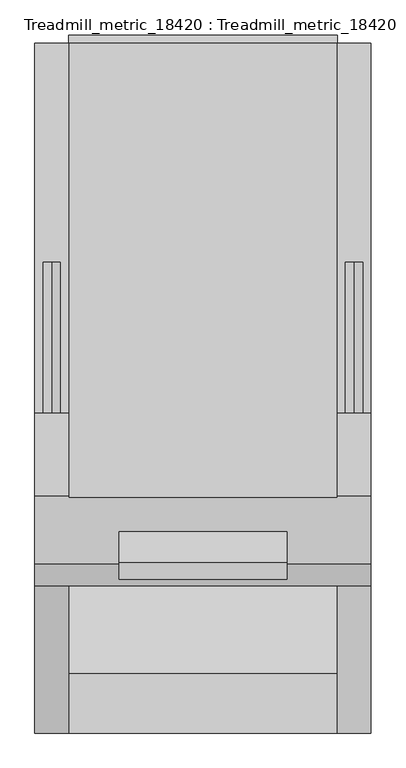
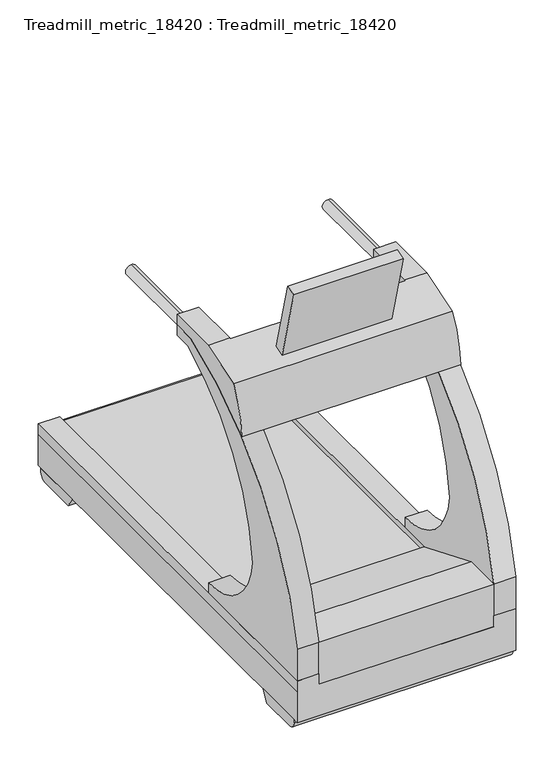
"""IFC4 building model written with IfcOpenShell, lengths in millimetres: proxy geometry, Treadmill_metric_18420 : Treadmill_metric_18420."""

from ifc_helpers import new_model, si_unit, point, frame, frame_2d, origin, place, context, project, spatial, polyline, circle_curve, trimmed, segment, composite_curve, outline, extrude, source, transform, mapped, element, save
from ifc_brep_helpers import plane_surface, cylinder_surface, revolved_surface, advanced_brep


def treadmill_metric_18420_treadmill_metric_18420_532483b1(model_context):
    return source(origin(), model_context, "Body", "SolidModel", [
        extrude(outline(composite_curve([segment(polyline([(1812.0655035, 0.0), (1781.1010673, 50.8), (2028.6449893, 50.8), (2028.6449893, 38.1)]), True, "CONTINUOUS"), segment(trimmed(circle_curve(frame_2d((1990.5449893, 38.1)), 38.1), [point((2028.6449893, 38.1))], [point((1990.5449893, 0.0))], False, "CARTESIAN"), True, "CONTINUOUS"), segment(polyline([(1990.5449893, 0.0), (1812.0655035, 0.0)]), True, "CONTINUOUS")], self_intersect=False)), frame((-136.4, 0.0, 0.0), z_axis=(1.0, 0.0, 0.0), x_axis=(0.0, 1.0, 0.0)), (0.0, 0.0, 1.0), 1000.0),
        extrude(outline(composite_curve([segment(polyline([(237.9344965, 0.0), (59.4550107, 0.0)]), True, "CONTINUOUS"), segment(trimmed(circle_curve(frame_2d((59.4550107, 38.1)), 38.1), [point((59.4550107, 0.0))], [point((21.3550107, 38.1))], False, "CARTESIAN"), True, "CONTINUOUS"), segment(polyline([(21.3550107, 38.1), (21.3550107, 50.8), (268.8989327, 50.8), (237.9344965, 0.0)]), True, "CONTINUOUS")], self_intersect=False)), frame((-136.4, 0.0, 0.0), z_axis=(1.0, 0.0, 0.0), x_axis=(0.0, 1.0, 0.0)), (0.0, 0.0, 1.0), 1000.0),
        extrude(outline(composite_curve([segment(trimmed(circle_curve(frame_2d((1371.6, -86.4)), 25.4), [point((1397.0, -86.4))], [point((1346.2, -86.4))], False, "CARTESIAN"), True, "CONTINUOUS"), segment(trimmed(circle_curve(frame_2d((1371.6, -86.4)), 25.4), [point((1346.2, -86.4))], [point((1397.0, -86.4))], False, "CARTESIAN"), True, "CONTINUOUS")], self_intersect=False)), frame((0.0, 950.0, 0.0), z_axis=(0.0, 1.0, 0.0), x_axis=(0.0, 0.0, 1.0)), (0.0, 0.0, 1.0), 450.0),
        extrude(outline(composite_curve([segment(trimmed(circle_curve(frame_2d((1371.6, 813.6)), 25.4), [point((1397.0, 813.6))], [point((1346.2, 813.6))], False, "CARTESIAN"), True, "CONTINUOUS"), segment(trimmed(circle_curve(frame_2d((1371.6, 813.6)), 25.4), [point((1346.2, 813.6))], [point((1397.0, 813.6))], False, "CARTESIAN"), True, "CONTINUOUS")], self_intersect=False)), frame((0.0, 950.0, 0.0), z_axis=(0.0, 1.0, 0.0), x_axis=(0.0, 0.0, 1.0)), (0.0, 0.0, 1.0), 450.0),
        extrude(outline(polyline([(200.0, -36.4), (250.8, -36.4), (250.8, -136.4), (200.0, -136.4), (50.8, -136.4), (50.8, 863.6), (200.0, 863.6), (250.8, 863.6), (250.8, 763.6), (200.0, 763.6), (200.0, -36.4)])), frame((0.0, 0.0, 0.0), z_axis=(0.0, 1.0, 0.0), x_axis=(0.0, 0.0, 1.0)), (0.0, 0.0, 1.0), 2050.0),
        extrude(outline(polyline([(550.0, 200.0), (0.0, 200.0), (0.0, 404.8), (177.8, 404.8), (550.0, 250.8), (550.0, 200.0)])), frame((-36.4, 0.0, 0.0), z_axis=(1.0, 0.0, 0.0), x_axis=(0.0, 1.0, 0.0)), (0.0, 0.0, 1.0), 800.0),
        extrude(outline(composite_curve([segment(polyline([(177.8, 200.0), (177.8, 225.4), (2050.0, 225.4)]), True, "CONTINUOUS"), segment(trimmed(circle_curve(frame_2d((2050.0, 200.0)), 25.4), [point((2050.0, 225.4))], [point((2050.0, 174.6))], False, "CARTESIAN"), True, "CONTINUOUS"), segment(polyline([(2050.0, 174.6), (2050.0, 200.0), (177.8, 200.0)]), True, "CONTINUOUS")], self_intersect=False)), frame((-36.4, 0.0, 0.0), z_axis=(1.0, 0.0, 0.0), x_axis=(0.0, 1.0, 0.0)), (0.0, 0.0, 1.0), 800.0),
        extrude(outline(composite_curve([segment(trimmed(circle_curve(frame_2d((1270.26111, 180.7492061)), 1289.8690034), [point((0.0, 404.8))], [point((840.7310736, 1397.0))], False, "CARTESIAN"), True, "CONTINUOUS"), segment(polyline([(840.7310736, 1397.0), (950.0, 1397.0), (950.0, 1346.2), (866.2507507, 1346.2)]), True, "CONTINUOUS"), segment(trimmed(circle_curve(frame_2d((1241.6021331, 534.0275676)), 894.7137644), [point((866.2507507, 1346.2))], [point((350.031958, 608.9631601))], True, "CARTESIAN"), True, "CONTINUOUS"), segment(trimmed(circle_curve(frame_2d((693.253891, 647.739532)), 345.4054174), [point((350.031958, 608.9631601))], [point((700.0, 302.4))], True, "CARTESIAN"), True, "CONTINUOUS"), segment(polyline([(700.0, 302.4), (700.0, 250.8), (0.0, 250.8), (0.0, 404.8)]), True, "CONTINUOUS")], self_intersect=False)), frame((-136.4, 0.0, 0.0), z_axis=(1.0, 0.0, 0.0), x_axis=(0.0, 1.0, 0.0)), (0.0, 0.0, 1.0), 100.0),
        extrude(outline(composite_curve([segment(trimmed(circle_curve(frame_2d((1270.26111, 180.7492061)), 1289.8690034), [point((0.0, 404.8))], [point((840.7310736, 1397.0))], False, "CARTESIAN"), True, "CONTINUOUS"), segment(polyline([(840.7310736, 1397.0), (950.0, 1397.0), (950.0, 1346.2), (866.2507507, 1346.2)]), True, "CONTINUOUS"), segment(trimmed(circle_curve(frame_2d((1241.6021331, 534.0275676)), 894.7137644), [point((866.2507507, 1346.2))], [point((350.031958, 608.9631601))], True, "CARTESIAN"), True, "CONTINUOUS"), segment(trimmed(circle_curve(frame_2d((693.253891, 647.739532)), 345.4054174), [point((350.031958, 608.9631601))], [point((700.0, 302.4))], True, "CARTESIAN"), True, "CONTINUOUS"), segment(polyline([(700.0, 302.4), (700.0, 250.8), (0.0, 250.8), (0.0, 404.8)]), True, "CONTINUOUS")], self_intersect=False)), frame((763.6, 0.0, 0.0), z_axis=(1.0, 0.0, 0.0), x_axis=(0.0, 1.0, 0.0)), (0.0, 0.0, 1.0), 100.0),
        advanced_brep(
        [(-136.4, 704.6599613, 1447.8), (-136.4, 950.0, 1447.8), (-136.4, 950.0, 1397.0), (-136.4, 840.7310736, 1397.0), (-136.4, 437.6082985, 1165.8640934), (-136.4, 501.9732306, 1384.2786219), (863.6, 704.6599613, 1447.8), (863.6, 501.9732306, 1384.2786219), (863.6, 437.6082985, 1165.8640934), (863.6, 840.7310736, 1397.0), (863.6, 950.0, 1397.0), (863.6, 950.0, 1447.8), (-36.4, 704.6599613, 1447.8), (-36.4, 950.0, 1447.8), (763.6, 950.0, 1447.8), (763.6, 704.6599613, 1447.8), (-36.4, 950.0, 1397.0), (763.6, 950.0, 1397.0), (-36.4, 840.7310736, 1397.0), (763.6, 840.7310736, 1397.0), (-36.4, 700.0, 1337.7126075), (763.6, 700.0, 1337.7126075), (763.6, 700.0, 1446.3395829), (-36.4, 700.0, 1446.3395829)],
        [
            (0, 1),
            (1, 2),
            (2, 3),
            (3, 4, circle_curve(frame((-136.4, 1270.26111, 180.7492061), z_axis=(1.0, 0.0, 0.0), x_axis=(0.0, 0.0, -1.0)), 1289.8690034)),
            (4, 5, circle_curve(frame((-136.4, 867.4146977, 1157.894915), z_axis=(-1.0, 0.0, 0.0), x_axis=(0.0, 0.0, -1.0)), 429.8802724)),
            (5, 0),
            (6, 7),
            (7, 8, circle_curve(frame((863.6, 867.4146977, 1157.894915), z_axis=(1.0, 0.0, 0.0), x_axis=(0.0, 0.0, -1.0)), 429.8802724)),
            (8, 9, circle_curve(frame((863.6, 1270.26111, 180.7492061), z_axis=(-1.0, 0.0, 0.0), x_axis=(0.0, 0.0, -1.0)), 1289.8690034)),
            (9, 10),
            (10, 11),
            (11, 6),
            (0, 12),
            (12, 13),
            (13, 1),
            (11, 14),
            (14, 15),
            (15, 6),
            (13, 16),
            (16, 2),
            (10, 17),
            (17, 14),
            (16, 18),
            (18, 3),
            (9, 19),
            (19, 17),
            (18, 20, circle_curve(frame((-36.4, 1270.26111, 180.7492061), z_axis=(1.0, 0.0, 0.0), x_axis=(0.0, 0.0, -1.0)), 1289.8690034)),
            (20, 21),
            (21, 19, circle_curve(frame((763.6, 1270.26111, 180.7492061), z_axis=(-1.0, 0.0, 0.0), x_axis=(0.0, 0.0, -1.0)), 1289.8690034)),
            (8, 4),
            (7, 5),
            (15, 22),
            (22, 23),
            (23, 12),
            (23, 20),
            (22, 21),
        ],
        [
            plane_surface(frame((-136.4, 1051.6662291, 1447.8), z_axis=(-1.0, 0.0, 0.0), x_axis=(0.0, 1.0, 0.0))),
            plane_surface(frame((863.6, 1051.6662291, 1447.8), z_axis=(1.0, 0.0, 0.0), x_axis=(0.0, -1.0, 0.0))),
            plane_surface(frame((-136.4, 704.6599613, 1447.8), z_axis=(0.0, 0.0, 1.0), x_axis=(1.0, 0.0, 0.0))),
            plane_surface(frame((-136.4, 950.0, 1447.8), z_axis=(0.0, 1.0, 0.0), x_axis=(1.0, 0.0, 0.0))),
            plane_surface(frame((-136.4, 950.0, 1397.0), z_axis=(0.0, 0.0, -1.0), x_axis=(1.0, 0.0, 0.0))),
            revolved_surface(polyline([(863.6, 1270.26111, -1109.1197973), (-136.39999999999998, 1270.26111, -1109.1197973)]), (863.6, 1270.26111, 180.7492061), (1.0, 0.0, 0.0)),
            cylinder_surface(frame((863.6, 867.4146977, 1157.894915), z_axis=(-1.0, 0.0, 0.0), x_axis=(0.0, 0.0, -1.0)), 429.8802724),
            plane_surface(frame((-136.4, 501.9732306, 1384.2786219), z_axis=(0.0, -0.29905454025397277, 0.9542360200461336), x_axis=(1.0, 0.0, 0.0))),
            plane_surface(frame((-36.4, 950.0, 1500.0), z_axis=(1.0, 0.0, 0.0), x_axis=(0.0, 0.0, -1.0))),
            plane_surface(frame((-36.4, 700.0, 1500.0), z_axis=(0.0, 1.0, 0.0), x_axis=(0.0, 0.0, -1.0))),
            plane_surface(frame((763.6, 700.0, 1500.0), z_axis=(-1.0, 0.0, 0.0), x_axis=(0.0, 0.0, -1.0))),
        ],
        [
            (0, [[1, 2, 3, 4, 5, 6]]),
            (1, [[7, 8, 9, 10, 11, 12]]),
            (2, [[-1, 13, 14, 15]]),
            (2, [[-12, 16, 17, 18]]),
            (3, [[-2, -15, 19, 20]]),
            (3, [[-11, 21, 22, -16]]),
            (4, [[-3, -20, 23, 24]]),
            (4, [[-10, 25, 26, -21]]),
            (5, [[-4, -24, 27, 28, 29, -25, -9, 30]]),
            (6, [[-5, -30, -8, 31]]),
            (7, [[-6, -31, -7, -18, 32, 33, 34, -13]]),
            (8, [[35, -27, -23, -19, -14, -34]]),
            (9, [[-35, -33, 36, -28]]),
            (10, [[-36, -32, -17, -22, -26, -29]]),
        ],
    ),
        extrude(outline(polyline([(0.0, -50.0), (0.0, 0.0), (500.0, 0.0), (500.0, -50.0), (0.0, -50.0)])), frame((113.6, 598.7271501, 1417.845423), z_axis=(0.0, -0.25881904510252135, 0.9659258262890681), x_axis=(1.0, 0.0, 0.0)), (0.0, 0.0, 1.0), 360.091105),
    ])


if __name__ == "__main__":
    model = new_model("IFC4")
    model_context = context("Model", 3, world=origin())
    ifc_project = project(units=[si_unit("LENGTHUNIT", "METRE", prefix="MILLI")], contexts=[model_context])
    site = spatial("IfcSite", under=ifc_project)
    building = spatial("IfcBuilding", under=site)
    placement = place(None, origin())
    treadmill_metric_18420_treadmill_metric_18420_shape = treadmill_metric_18420_treadmill_metric_18420_532483b1(model_context)
    element("IfcBuildingElementProxy", 1, Name="Treadmill_metric_18420 : Treadmill_metric_18420", ObjectType="Treadmill_metric_18420 : Treadmill_metric_18420", at=placement, inside=building, context=model_context, shape_type="MappedRepresentation", body=[
        mapped(treadmill_metric_18420_treadmill_metric_18420_shape, transform((0.0, 0.0, 0.0), x_axis=(1.0, 0.0, 0.0), y_axis=(0.0, 1.0, 0.0), z_axis=(0.0, 0.0, 1.0))),
    ])
    save(model, "model.ifc")

# Revit data of these elements
# Type "Treadmill_metric_18420 : Treadmill_metric_18420"
#   Assembly Code = "E1090"
#   width = 3' - 3.37008"
#   belt width = 2' - 7.49606"
#   Lenght = 6' - 8.70866"
#   Default Elevation = 0
# Element 1 (IfcBuildingElementProxy, "Treadmill_metric_18420 : Treadmill_metric_18420")
#   Materials on its faces: "Metal - Steel", "Default"
# Materials
#   "Metal - Steel": colour RGB 247 247 247, transparency 0
#   "Default": colour RGB 127 127 127, transparency 0, Cost = 0
